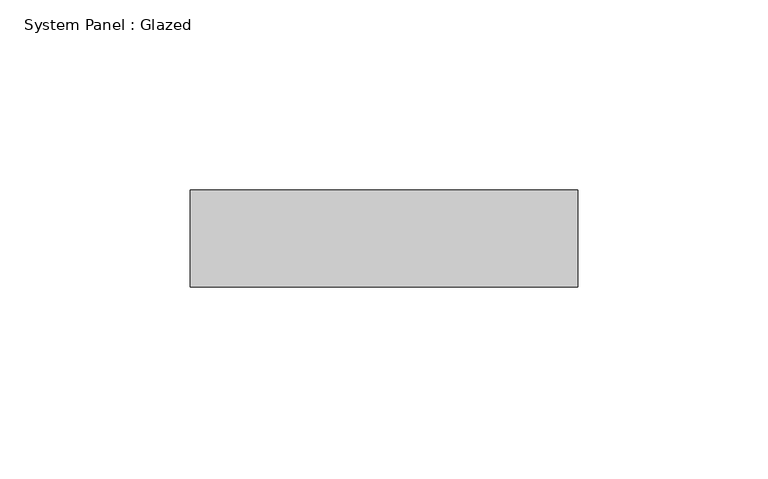
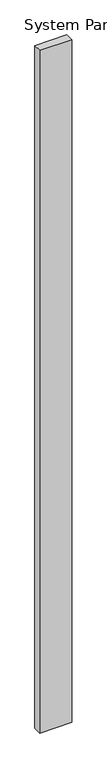
"""IFC4 building model written with IfcOpenShell, lengths in millimetres: plate geometry, System Panel : Glazed."""

from ifc_helpers import new_model, si_unit, origin, origin_with_axes, place, context, project, spatial, polyline, outline, extrude, source, transform, mapped, element, save


def system_panel_glazed_28c5fff6(model_context):
    return source(origin(), model_context, "Body", "SweptSolid", [
        extrude(outline(polyline([(50.8, 19.05), (-50.8, 19.05), (-50.8, 44.45), (50.8, 44.45), (50.8, 19.05)])), origin_with_axes(), (0.0, 0.0, 1.0), 2287.5875),
    ])


if __name__ == "__main__":
    model = new_model("IFC4")
    model_context = context("Model", 3, world=origin())
    ifc_project = project(units=[si_unit("LENGTHUNIT", "METRE", prefix="MILLI")], contexts=[model_context])
    site = spatial("IfcSite", under=ifc_project)
    building = spatial("IfcBuilding", under=site)
    placement = place(None, origin())
    system_panel_glazed_shape = system_panel_glazed_28c5fff6(model_context)
    element("IfcPlate", 1, ObjectType="System Panel : Glazed", at=placement, inside=building, context=model_context, shape_type="MappedRepresentation", body=[
        mapped(system_panel_glazed_shape, transform((0.0, 0.0, 0.0), x_axis=(1.0, 0.0, 0.0), y_axis=(0.0, 1.0, 0.0), z_axis=(0.0, 0.0, 1.0))),
    ])
    save(model, "model.ifc")

# Revit data of these elements
# Type "System Panel : Glazed"
#   Construction Type Id = "GSP4R"
#   Analytic Construction = "1/8 in Pilkington single glazing"
#   Visual Light Transmittance = 0.9
#   Solar Heat Gain Coefficient = 0.86
#   Heat Transfer Coefficient (U) = 1.18115 BTU/(h·ft²·°F)
#   Define Thermal Properties by = 1
# Element 1 (IfcPlate, "System Panel : Glazed")
#   Materials on its faces: "Glass"
# Materials
#   "Glass": class "Glass", colour RGB 0 128 192, transparency 0.75, Description = "Soda Lime Glass", Cost = 0
